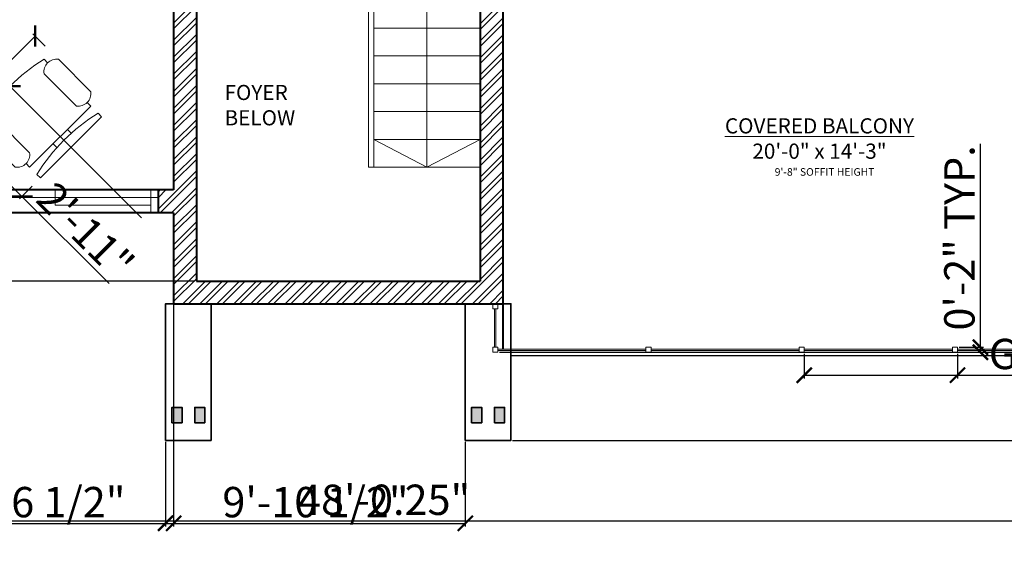
# Model space of a CAD drawing. Units: inches. Extents: x 982 to 1904, y 735 to 1463.
# Tile 2 of 7: x 1301 to 1689, y 735 to 945. Entities that reach past the tile are written whole.
import ezdxf

# ---------------------------------------------------------------- set-up
doc = ezdxf.new("R2010")
doc.units = ezdxf.units.IN
for name, color, linetype, lineweight in [('A-ANNO-TEXT', 7, 'Continuous', 18), ('A-AREA-IDEN', 7, 'Continuous', 18), ('A-COLS', 7, 'Continuous', 35), ('A-FLOR', 7, 'Continuous', 25), ('A-FLOR-RAIL', 7, 'Continuous', 18), ('Dimensions', 9, 'Continuous', 18), ('Furniture', 31, 'Continuous', 18), ('Stairs', 50, 'Continuous', 20), ('Wall Hatch', 23, 'Continuous', 13), ('Walls', 151, 'Continuous', 40), ('Windows', 111, 'Continuous', 18)]:
    doc.layers.add(name, color=color, linetype=linetype, lineweight=lineweight)
doc.layers.add('A-COLS-PATT', color=251, linetype='Continuous', lineweight=13, true_color=0x636466)
doc.styles.get("Standard").update_dxf_attribs({"font": 'arial.ttf'})
doc.dimstyles.new('ISO-25', dxfattribs={"dimtxt": 12, "dimasz": 6, "dimexe": 1.25, "dimexo": 0.625, "dimtad": 1, "dimlunit": 3, "dimtxsty": 'Standard', "dimblk": 'ARCHTICK', "dimcen": 2.5, "dimadec": 0, "dimazin": 0, "dimtfac": 1, "dimtmove": 0, "dimatfit": 3, "dimfxl": 1, "dimarcsym": 0})

# ---------------------------------------------------------------- blocks, each defined once
blk = doc.blocks.new('Chair - Desk')
for p, q in [((-8.5, 0), (-8.5, -1)), ((-8.5, 0), (8.5, 0)), ((8.5, 0), (8.5, -1)), ((-8.5, -3), (-8.5, -4)), ((-8.5, -3), (8.5, -3)), ((-2, -3), (-2, -1.9355)), ((2, -1.9576), (2, -3)), ((8.5, -3), (8.5, -4)), ((-10.5, -5), (-10.5, -14)), ((-6.5, -14), (-6.5, -5)), ((6.5, -5), (6.5, -14)), ((10.5, -14), (10.5, -5)), ((-8.5, -15), (-8.5, -16)), ((8.5, -15), (8.5, -16))]:
    blk.add_line(p, q)
for centre, radius, start, end in [((0, 34.625), 36.625, 256.5803, 283.4197), ((-8.5, -6.5), 2.5, 36.8699, 143.1301), ((8.5, -6.5), 2.5, 36.8699, 143.1301), ((-8.5, -12.5), 2.5, 216.8699, 323.1301), ((8.5, -12.5), 2.5, 216.8699, 323.1301), ((0, 19.625), 36.625, 256.5803, 283.4197)]:
    blk.add_arc(centre, radius, start, end)
blk = doc.blocks.new('_ArchTick')
at = {"color": 0, "linetype": 'ByBlock', "const_width": 0.15}
blk.add_lwpolyline([(-0.5, -0.5), (0.5, 0.5)], dxfattribs=at)
blk = doc.blocks.new('*D22')
at = {"layer": 'Defpoints', "color": 0, "transparency": 16777216}
for p in [(1156.5, 893.99), (1732.75, 812.49), (1732.75, 747.2)]:
    blk.add_point(p, dxfattribs=at)
at = {"layer": 'Dimensions', "color": 0, "lineweight": -2, "transparency": 16777216}
for p, q in [((1156.5, 893.37), (1156.5, 745.95)), ((1732.75, 811.87), (1732.75, 745.95)), ((1156.5, 747.2), (1732.75, 747.2))]:
    blk.add_line(p, q, dxfattribs=at)
at = {"layer": 'Dimensions', "color": 0, "lineweight": -2, "transparency": 16777216, "xscale": 6, "yscale": 6, "zscale": 6, "rotation": 180}
blk.add_blockref('_ArchTick', (1156.5, 747.2), dxfattribs=at)
at = {"layer": 'Dimensions', "color": 0, "lineweight": -2, "transparency": 16777216, "xscale": 6, "yscale": 6, "zscale": 6}
blk.add_blockref('_ArchTick', (1732.75, 747.2), dxfattribs=at)
at = {"layer": 'Dimensions', "color": 0, "transparency": 16777216, "insert": (1444.62, 753.95), "char_height": 12, "attachment_point": 5}
blk.add_mtext('48\'-0.25"', dxfattribs=at)
blk = doc.blocks.new('POST-BASE-18x54')
for points in [[(0, 0), (18, 0), (18, 54), (0, 54)], [(2.5, 7), (6.5, 7), (6.5, 13), (2.5, 13)], [(11.5, 7), (15.5, 7), (15.5, 13), (11.5, 13)]]:
    blk.add_lwpolyline(points, close=True)
blk = doc.blocks.new('GUARD-PANEL-60_5')
for p, q in [((0, 1.16), (58.5, 1.16)), ((0, 0.66), (58.5, 0.66))]:
    blk.add_line(p, q)
blk.add_lwpolyline([(58.5, 2), (60.5, 2), (60.5, 0), (58.5, 0)], close=True)
blk = doc.blocks.new('*D28')
at = {"layer": 'Defpoints', "color": 0, "transparency": 16777216}
for p in [(1610.5, 813.83), (1671, 813.83), (1671, 804.76)]:
    blk.add_point(p, dxfattribs=at)
at = {"layer": 'Dimensions', "color": 0, "lineweight": -2, "transparency": 16777216}
for p, q in [((1610.5, 813.21), (1610.5, 803.51)), ((1671, 813.21), (1671, 803.51)), ((1610.5, 804.76), (1671, 804.76)), ((1671, 804.76), (1903.99, 804.76))]:
    blk.add_line(p, q, dxfattribs=at)
at = {"layer": 'Dimensions', "color": 0, "lineweight": -2, "transparency": 16777216, "xscale": 6, "yscale": 6, "zscale": 6, "rotation": 180}
blk.add_blockref('_ArchTick', (1610.5, 804.76), dxfattribs=at)
at = {"layer": 'Dimensions', "color": 0, "lineweight": -2, "transparency": 16777216, "xscale": 6, "yscale": 6, "zscale": 6}
blk.add_blockref('_ArchTick', (1671, 804.76), dxfattribs=at)
at = {"layer": 'Dimensions', "color": 0, "transparency": 16777216, "insert": (1790.49, 811.59), "char_height": 12, "attachment_point": 5}
blk.add_mtext('GUARD PANEL 5\'-0 1/2" TYP.', dxfattribs=at)
blk = doc.blocks.new('*D29')
at = {"layer": 'Defpoints', "color": 0, "transparency": 16777216}
for p in [(1671, 815.83), (1671, 813.83), (1680.07, 815.83)]:
    blk.add_point(p, dxfattribs=at)
at = {"layer": 'Dimensions', "color": 0, "lineweight": -2, "transparency": 16777216}
for p, q in [((1680.07, 815.83), (1680.07, 896.23)), ((1671.62, 815.83), (1681.32, 815.83)), ((1671.62, 813.83), (1681.32, 813.83)), ((1680.07, 813.83), (1680.07, 815.83))]:
    blk.add_line(p, q, dxfattribs=at)
at = {"layer": 'Dimensions', "color": 0, "lineweight": -2, "transparency": 16777216, "xscale": 6, "yscale": 6, "zscale": 6}
for p, rotation in [((1680.07, 815.83), 90), ((1680.07, 813.83), 270)]:
    blk.add_blockref('_ArchTick', p, dxfattribs=dict(at, rotation=rotation))
at = {"layer": 'Dimensions', "color": 0, "transparency": 16777216, "insert": (1673.32, 859.03), "char_height": 12, "attachment_point": 5, "rotation": 90}
blk.add_mtext('0\'-2" TYP.', dxfattribs=at)
blk = doc.blocks.new('*D50')
at = {"layer": 'Defpoints', "color": 0, "transparency": 16777216}
for p in [(1311.27, 934.37), (1276.96, 909.01), (1281.43, 904.53)]:
    blk.add_point(p, dxfattribs=at)
at = {"layer": 'Dimensions', "color": 0, "lineweight": -2, "transparency": 16777216}
for p, q in [((1306.8, 938.85), (1276.96, 909.01)), ((1310.83, 934.81), (1305.91, 939.73)), ((1280.99, 904.97), (1276.07, 909.89)), ((1276.96, 909.01), (1173.95, 806))]:
    blk.add_line(p, q, dxfattribs=at)
at = {"layer": 'Dimensions', "color": 0, "lineweight": -2, "transparency": 16777216, "xscale": 6, "yscale": 6, "zscale": 6}
for p, rotation in [((1306.8, 938.85), 44.99970894708495), ((1276.96, 909.01), 224.9997089470849)]:
    blk.add_blockref('_ArchTick', p, dxfattribs=dict(at, rotation=rotation))
at = {"layer": 'Dimensions', "color": 0, "transparency": 16777216, "insert": (1218.5, 860.22), "char_height": 12, "attachment_point": 5, "rotation": 44.9997}
blk.add_mtext('DESK CHAIR 3\'-6"', dxfattribs=at)
blk = doc.blocks.new('*D51')
at = {"layer": 'Defpoints', "color": 0, "transparency": 16777216}
for p in [(1281.43, 904.53), (1306.06, 879.9), (1301.59, 875.42)]:
    blk.add_point(p, dxfattribs=at)
at = {"layer": 'Dimensions', "color": 0, "lineweight": -2, "transparency": 16777216}
for p, q in [((1280.99, 904.09), (1276.07, 899.17)), ((1276.96, 900.06), (1301.59, 875.42)), ((1305.62, 879.46), (1300.7, 874.54)), ((1301.59, 875.42), (1336.01, 841))]:
    blk.add_line(p, q, dxfattribs=at)
at = {"layer": 'Dimensions', "color": 0, "lineweight": -2, "transparency": 16777216, "xscale": 6, "yscale": 6, "zscale": 6}
for p, rotation in [((1276.96, 900.06), 134.9997089470847), ((1301.59, 875.42), 314.9997089470847)]:
    blk.add_blockref('_ArchTick', p, dxfattribs=dict(at, rotation=rotation))
at = {"layer": 'Dimensions', "color": 0, "transparency": 16777216, "insert": (1325.62, 860.8), "char_height": 12, "attachment_point": 5, "rotation": 314.9997}
blk.add_mtext('2\'-11"', dxfattribs=at)
blk = doc.blocks.new('*D54')
at = {"layer": 'Defpoints', "color": 0, "transparency": 16777216}
for p in [(1489.5, 813.83), (1769.32, 813.83), (1494.68, 778.99)]:
    blk.add_point(p, dxfattribs=at)
at = {"layer": 'Dimensions', "color": 0, "lineweight": -2, "transparency": 16777216}
for p, q in [((1769.32, 813.83), (1769.32, 862.51)), ((1490.12, 813.83), (1770.57, 813.83)), ((1769.32, 778.99), (1769.32, 813.83)), ((1495.3, 778.99), (1770.57, 778.99))]:
    blk.add_line(p, q, dxfattribs=at)
at = {"layer": 'Dimensions', "color": 0, "lineweight": -2, "transparency": 16777216, "xscale": 6, "yscale": 6, "zscale": 6}
for p, rotation in [((1769.32, 813.83), 90), ((1769.32, 778.99), 270)]:
    blk.add_blockref('_ArchTick', p, dxfattribs=dict(at, rotation=rotation))
at = {"layer": 'Dimensions', "color": 0, "transparency": 16777216, "insert": (1762.67, 841.17), "char_height": 12, "attachment_point": 5, "rotation": 90}
blk.add_mtext('2\'-11"', dxfattribs=at)
blk = doc.blocks.new('*D62')
at = {"layer": 'Defpoints', "color": 0, "transparency": 16777216}
for p in [(1259, 868.99), (1361.5, 868.99), (1361.5, 746.19)]:
    blk.add_point(p, dxfattribs=at)
at = {"layer": 'Dimensions', "color": 0, "lineweight": -2, "transparency": 16777216}
for p, q in [((1259, 868.37), (1259, 744.94)), ((1361.5, 868.37), (1361.5, 744.94)), ((1259, 746.19), (1361.5, 746.19))]:
    blk.add_line(p, q, dxfattribs=at)
at = {"layer": 'Dimensions', "color": 0, "lineweight": -2, "transparency": 16777216, "xscale": 6, "yscale": 6, "zscale": 6, "rotation": 180}
blk.add_blockref('_ArchTick', (1259, 746.19), dxfattribs=at)
at = {"layer": 'Dimensions', "color": 0, "lineweight": -2, "transparency": 16777216, "xscale": 6, "yscale": 6, "zscale": 6}
blk.add_blockref('_ArchTick', (1361.5, 746.19), dxfattribs=at)
at = {"layer": 'Dimensions', "color": 0, "transparency": 16777216, "insert": (1310.25, 753.02), "char_height": 12, "attachment_point": 5}
blk.add_mtext('8\'-6 1/2"', dxfattribs=at)
blk = doc.blocks.new('*D64')
at = {"layer": 'Defpoints', "color": 0, "transparency": 16777216}
for p in [(1482.5, 1427.79), (1370.5, 841.99), (1482.5, 841.99)]:
    blk.add_point(p, dxfattribs=at)
at = {"layer": 'Dimensions', "color": 0, "lineweight": -2, "transparency": 16777216}
for p, q in [((1370.5, 842.62), (1370.5, 1429.04)), ((1370.5, 1427.79), (1482.5, 1427.79)), ((1482.5, 842.62), (1482.5, 1429.04))]:
    blk.add_line(p, q, dxfattribs=at)
at = {"layer": 'Dimensions', "color": 0, "lineweight": -2, "transparency": 16777216, "xscale": 6, "yscale": 6, "zscale": 6, "rotation": 180}
blk.add_blockref('_ArchTick', (1370.5, 1427.79), dxfattribs=at)
at = {"layer": 'Dimensions', "color": 0, "lineweight": -2, "transparency": 16777216, "xscale": 6, "yscale": 6, "zscale": 6}
blk.add_blockref('_ArchTick', (1482.5, 1427.79), dxfattribs=at)
at = {"layer": 'Dimensions', "color": 0, "transparency": 16777216, "insert": (1426.5, 1434.54), "char_height": 12, "attachment_point": 5}
blk.add_mtext('9\'-4"', dxfattribs=at)
blk = doc.blocks.new('*D65')
at = {"layer": 'Defpoints', "color": 0, "transparency": 16777216}
for p in [(1123.7, 1042.99), (1370.5, 1042.99), (1370.5, 841.99)]:
    blk.add_point(p, dxfattribs=at)
at = {"layer": 'Dimensions', "color": 0, "lineweight": -2, "transparency": 16777216}
for p, q in [((1369.87, 1042.99), (1122.45, 1042.99)), ((1123.7, 841.99), (1123.7, 1042.99)), ((1369.87, 841.99), (1122.45, 841.99))]:
    blk.add_line(p, q, dxfattribs=at)
at = {"layer": 'Dimensions', "color": 0, "lineweight": -2, "transparency": 16777216, "xscale": 6, "yscale": 6, "zscale": 6}
for p, rotation in [((1123.7, 1042.99), 90), ((1123.7, 841.99), 270)]:
    blk.add_blockref('_ArchTick', p, dxfattribs=dict(at, rotation=rotation))
at = {"layer": 'Dimensions', "color": 0, "transparency": 16777216, "insert": (1116.94, 942.49), "char_height": 12, "attachment_point": 5, "rotation": 90}
blk.add_mtext('16\'-9"', dxfattribs=at)
blk = doc.blocks.new('*D71')
at = {"layer": 'Defpoints', "color": 0, "transparency": 16777216}
for p in [(1358.31, 778.99), (1476.68, 778.99), (1476.68, 746.19)]:
    blk.add_point(p, dxfattribs=at)
at = {"layer": 'Dimensions', "color": 0, "lineweight": -2, "transparency": 16777216}
for p, q in [((1358.31, 778.37), (1358.31, 744.94)), ((1476.68, 778.37), (1476.68, 744.94)), ((1358.31, 746.19), (1476.68, 746.19))]:
    blk.add_line(p, q, dxfattribs=at)
at = {"layer": 'Dimensions', "color": 0, "lineweight": -2, "transparency": 16777216, "xscale": 6, "yscale": 6, "zscale": 6, "rotation": 180}
blk.add_blockref('_ArchTick', (1358.31, 746.19), dxfattribs=at)
at = {"layer": 'Dimensions', "color": 0, "lineweight": -2, "transparency": 16777216, "xscale": 6, "yscale": 6, "zscale": 6}
blk.add_blockref('_ArchTick', (1476.68, 746.19), dxfattribs=at)
at = {"layer": 'Dimensions', "color": 0, "transparency": 16777216, "insert": (1417.5, 753.02), "char_height": 12, "attachment_point": 5}
blk.add_mtext('9\'-10 1/2"', dxfattribs=at)
blk = doc.blocks.new('*D75')
at = {"layer": 'Defpoints', "color": 0, "transparency": 16777216}
for p in [(1296.83, 918.98), (1348.87, 866.93)]:
    blk.add_point(p, dxfattribs=at)
at = {"layer": 'Dimensions', "color": 0, "lineweight": -2, "transparency": 16777216}
for p in [(1218.63, 997.17), (1348.87, 866.93)]:
    blk.add_line(p, (1296.83, 918.98), dxfattribs=at)
at = {"layer": 'Dimensions', "color": 0, "lineweight": -2, "transparency": 16777216, "xscale": 6, "yscale": 6, "zscale": 6, "rotation": 314.9994011111431}
blk.add_blockref('_ArchTick', (1296.83, 918.98), dxfattribs=at)
at = {"layer": 'Dimensions', "color": 0, "transparency": 16777216, "insert": (1258.32, 967.15), "char_height": 12, "attachment_point": 5, "rotation": 314.9994}
blk.add_mtext('2X R6\'-1 1/2"', dxfattribs=at)

msp = doc.modelspace()

# ---------------------------------------------------------------- hatches: boundary and pattern name
at = {"layer": 'A-COLS-PATT'}
h = msp.add_hatch(color=256, dxfattribs=at)
h.dxf.hatch_style = 1
h.paths.add_polyline_path([(1731.496, 1394.991), (1722.496, 1394.991), (1722.496, 1385.991), (1731.496, 1385.991)])
h.paths.add_polyline_path([(1725.019, 843.656), (1721.019, 843.656), (1721.019, 837.656), (1725.019, 837.656)])
h.paths.add_polyline_path([(1734.019, 843.656), (1730.019, 843.656), (1730.019, 837.656), (1734.019, 837.656)])
h.paths.add_polyline_path([(1483.18, 791.991), (1479.18, 791.991), (1479.18, 785.991), (1483.18, 785.991)])
h.paths.add_polyline_path([(1492.18, 791.991), (1488.18, 791.991), (1488.18, 785.991), (1492.18, 785.991)])
h.paths.add_polyline_path([(1364.813, 791.991), (1360.813, 791.991), (1360.813, 785.991), (1364.813, 785.991)])
h.paths.add_polyline_path([(1373.813, 791.991), (1369.813, 791.991), (1369.813, 785.991), (1373.813, 785.991)])
at = {"layer": 'Wall Hatch'}
h = msp.add_hatch(dxfattribs=at)
h.set_pattern_fill('ANSI32', color=256, scale=0.5)
h.paths.add_polyline_path([(1165.496, 1065.991), (1271.496, 1065.991), (1271.496, 1071.991), (1218.496, 1071.991), (1218.496, 1238.491), (1262.496, 1238.491), (1262.496, 1244.491), (1218.496, 1244.491), (1218.496, 1330.491), (1298.496, 1330.491), (1298.496, 1244.491), (1292.496, 1244.491), (1292.496, 1238.491), (1298.496, 1238.491), (1298.496, 1221.991), (1304.496, 1221.991), (1304.496, 1224.991), (1374.496, 1224.991), (1374.496, 1230.991), (1304.496, 1230.991), (1304.496, 1251.991), (1310.496, 1251.991), (1310.496, 1257.991), (1304.496, 1257.991), (1304.496, 1385.991), (1328.496, 1385.991), (1328.496, 1394.991), (1295.496, 1394.991), (1295.496, 1339.491), (1209.496, 1339.491), (1209.496, 1071.991), (1156.496, 1071.991), (1156.496, 893.991), (1171.496, 893.991), (1171.496, 902.991), (1165.496, 902.991)])
h.paths.add_polyline_path([(1273.996, 877.991), (1267.996, 877.991), (1267.996, 902.991), (1252.996, 902.991), (1252.996, 893.991), (1258.996, 893.991), (1258.996, 868.991), (1273.996, 868.991)])
h.paths.add_polyline_path([(1370.496, 1052.991), (1361.496, 1052.991), (1361.496, 1046.991), (1355.496, 1046.991), (1355.496, 1040.991), (1361.496, 1040.991), (1361.496, 877.991), (1355.496, 877.991), (1355.496, 868.991), (1361.496, 868.991), (1361.496, 832.991), (1376.313, 832.991), (1491.496, 832.991), (1491.496, 985.991), (1515.496, 985.991), (1515.496, 994.991), (1482.496, 994.991), (1482.496, 841.991), (1370.496, 841.991)])
h.paths.add_polyline_path([(1319.496, 1088.991), (1325.496, 1088.991), (1325.496, 1094.991), (1319.496, 1094.991), (1319.496, 1112.491), (1361.496, 1112.491), (1361.496, 1094.991), (1355.496, 1094.991), (1355.496, 1088.991), (1361.496, 1088.991), (1361.496, 1082.991), (1370.496, 1082.991), (1370.496, 1180.991), (1503.496, 1180.991), (1503.496, 1231.991), (1497.496, 1231.991), (1497.496, 1215.991), (1491.496, 1215.991), (1491.496, 1209.991), (1497.496, 1209.991), (1497.496, 1189.991), (1448.496, 1189.991), (1448.496, 1209.991), (1454.496, 1209.991), (1454.496, 1215.991), (1448.496, 1215.991), (1448.496, 1221.991), (1442.496, 1221.991), (1442.496, 1189.991), (1380.496, 1189.991), (1380.496, 1251.991), (1442.496, 1251.991), (1442.496, 1245.991), (1448.496, 1245.991), (1448.496, 1263.991), (1442.496, 1263.991), (1442.496, 1257.991), (1368.496, 1257.991), (1368.496, 1251.991), (1374.496, 1251.991), (1374.496, 1189.991), (1304.496, 1189.991), (1304.496, 1192.991), (1295.496, 1192.991), (1295.496, 1183.991), (1361.496, 1183.991), (1361.496, 1118.491), (1313.496, 1118.491), (1313.496, 1071.991), (1301.496, 1071.991), (1301.496, 1065.991), (1313.496, 1065.991), (1313.496, 1040.991), (1325.496, 1040.991), (1325.496, 1046.991), (1319.496, 1046.991)])
h.paths.add_polyline_path([(1565.496, 1394.991), (1418.496, 1394.991), (1418.496, 1385.991), (1442.496, 1385.991), (1442.496, 1293.991), (1448.496, 1293.991), (1448.496, 1299.991), (1454.496, 1299.991), (1454.496, 1305.991), (1448.496, 1305.991), (1448.496, 1385.991), (1556.496, 1385.991), (1556.496, 1307.991), (1497.496, 1307.991), (1497.496, 1305.991), (1491.496, 1305.991), (1491.496, 1299.991), (1497.496, 1299.991), (1497.496, 1268.991), (1503.496, 1268.991), (1503.496, 1298.991), (1656.496, 1298.991), (1656.496, 1307.991), (1565.496, 1307.991)])
h.paths.add_polyline_path([(1731.496, 1307.991), (1698.496, 1307.991), (1698.496, 1298.991), (1722.496, 1298.991), (1722.496, 1033.991), (1731.496, 1033.991)])
h.paths.add_polyline_path([(1731.496, 997.991), (1722.496, 997.991), (1722.496, 994.991), (1689.496, 994.991), (1689.496, 985.991), (1731.496, 985.991)])

# ---------------------------------------------------------------- linework, layer by layer
at = {"layer": 'A-FLOR'}
msp.add_line((1494.68, 812.491), (1732.746, 812.491), dxfattribs=at)
at = {"layer": 'A-FLOR-RAIL'}
for p, q in [((1488.246, 830.991), (1488.246, 815.833)), ((1488.746, 830.991), (1488.746, 815.833))]:
    msp.add_line(p, q, dxfattribs=at)
for points in [[(1487.496, 830.991), (1489.496, 830.991), (1489.496, 832.991), (1487.496, 832.991)], [(1487.496, 815.833), (1489.496, 815.833), (1489.496, 813.833), (1487.496, 813.833)]]:
    msp.add_lwpolyline(points, close=True, dxfattribs=at)
at = {"layer": 'Stairs'}
for p, q in [((1438.496, 1043.012), (1438.496, 886.991)), ((1440.496, 1043.012), (1440.496, 886.991)), ((1461.496, 886.991), (1461.496, 1043.019)), ((1440.496, 941.991), (1482.496, 941.991)), ((1440.496, 930.991), (1482.496, 930.991)), ((1440.496, 919.991), (1482.496, 919.991)), ((1440.496, 908.991), (1482.496, 908.991)), ((1440.496, 897.991), (1482.496, 897.991)), ((1440.496, 897.991), (1461.496, 886.991)), ((1461.496, 886.991), (1482.496, 897.991)), ((1438.496, 886.991), (1482.496, 886.991))]:
    msp.add_line(p, q, dxfattribs=at)
at = {"layer": 'Walls'}
for p, q in [((1370.496, 1052.991), (1370.496, 841.991)), ((1482.496, 1043.025), (1482.496, 841.991)), ((1361.496, 1040.991), (1361.496, 877.991)), ((1491.496, 985.991), (1491.496, 814.991)), ((1361.496, 877.991), (1267.996, 877.991)), ((1355.496, 868.991), (1355.496, 877.991)), ((1361.496, 868.991), (1258.996, 868.991)), ((1361.496, 868.991), (1361.496, 832.991)), ((1370.496, 841.991), (1482.496, 841.991)), ((1361.496, 832.991), (1491.496, 832.991))]:
    msp.add_line(p, q, dxfattribs=at)
at = {"layer": 'Windows'}
for p, q in [((1355.496, 874.991), (1273.996, 874.991)), ((1314.746, 877.991), (1314.746, 871.991)), ((1352.496, 868.991), (1352.496, 877.991)), ((1352.496, 871.991), (1314.746, 871.991))]:
    msp.add_line(p, q, dxfattribs=at)

# ---------------------------------------------------------------- block references
at = {"layer": 'A-COLS', "extrusion": (0, 0, -1), "zscale": -1}
msp.add_blockref('POST-BASE-18x54', (-1376.313, 778.991), dxfattribs=at)
at = {"layer": 'A-COLS'}
msp.add_blockref('POST-BASE-18x54', (1476.68, 778.991), dxfattribs=at)
at = {"layer": 'A-FLOR-RAIL'}
for p in [(1489.496, 813.833), (1549.996, 813.833), (1610.496, 813.833), (1670.996, 813.833)]:
    msp.add_blockref('GUARD-PANEL-60_5', p, dxfattribs=at)
at = {"layer": 'Furniture', "xscale": 2.009614080572303, "yscale": 2.009614080572303, "zscale": 2.009614080572303, "rotation": 224.9997089470848}
msp.add_blockref('Chair - Desk', (1320.983, 894.821), dxfattribs=at)

# ---------------------------------------------------------------- texts
at = {"layer": 'A-ANNO-TEXT', "insert": (1575.903, 886.614), "char_height": 3, "attachment_point": 1}
msp.add_mtext_dynamic_manual_height_columns('\\pxqc;{\\fTimes New Roman|b0|i0|c0|p18;\\T1.25;9\'-8" SOFFIT HEIGHT}', width=85.22884, gutter_width=12.5, heights=[0], dxfattribs=at)
at = {"layer": 'A-AREA-IDEN', "char_height": 6, "attachment_point": 1}
for s, width, insert in [('{\\fTimes New Roman|b0|i0|c0|p18;FOYER BELOW}', 41.80763, (1381.603, 919.526)), ('\\pxqc;{\\fTimes New Roman|b0|i0|c0|p18;\\LCOVERED BALCONY\\P\\l20\'-0" x 14\'-3"}', 97.93162, (1567.548, 906.326))]:
    msp.add_mtext_dynamic_manual_height_columns(s, width=width, gutter_width=12.5, heights=[0], dxfattribs=dict(at, insert=insert))

# ---------------------------------------------------------------- dimensions: what is measured, and where the dimension line sits
at = {"layer": 'Dimensions'}
for base, p1, p2, override, picture, middle in [((1482.496, 1427.791), (1370.496, 841.991), (1482.496, 841.991), {"dimdec": 1, "dimlfac": 1, "dimrnd": 0, "dimzin": 1, "dimdsep": 46, "dimlunit": 4, "dimfrac": 2}, '*D64', (1426.496, 1434.543)), ((1732.746, 747.196), (1156.496, 893.991), (1732.746, 812.491), {"dimclrd": 0, "dimclre": 0, "dimclrt": 0}, '*D22', (1444.621, 753.948)), ((1361.496, 746.191), (1258.996, 868.991), (1361.496, 868.991), {"dimdec": 1, "dimlfac": 1, "dimrnd": 0, "dimzin": 1, "dimdsep": 46, "dimlunit": 4, "dimfrac": 2}, '*D62', (1310.246, 753.021)), ((1476.68, 746.191), (1358.313, 778.991), (1476.68, 778.991), {"dimdec": 1, "dimlfac": 1, "dimrnd": 0, "dimzin": 1, "dimdsep": 46, "dimlunit": 4, "dimfrac": 2}, '*D71', (1417.496, 753.021))]:
    dim = msp.add_linear_dim(base=base, p1=p1, p2=p2, dimstyle='ISO-25', override=override, dxfattribs=at)
    dim.commit()
    dim.dimension.update_dxf_attribs({"geometry": picture, "text_midpoint": middle})
for base, p1, p2, angle, picture, middle in [((1123.696, 1042.991), (1370.496, 841.991), (1370.496, 1042.991), 90, '*D65', (1116.945, 942.491)), ((1301.586, 875.425), (1281.431, 904.532), (1306.062, 879.901), 314.99971, '*D51', (1325.619, 860.795)), ((1769.319, 813.833), (1494.68, 778.991), (1489.496, 813.833), 90, '*D54', (1762.669, 841.172))]:
    dim = msp.add_linear_dim(base=base, p1=p1, p2=p2, angle=angle, dimstyle='ISO-25', override={"dimdec": 1, "dimlfac": 1, "dimrnd": 0, "dimzin": 1, "dimdsep": 46, "dimlunit": 4, "dimfrac": 2}, dxfattribs=at)
    dim.commit()
    dim.dimension.update_dxf_attribs({"geometry": picture, "text_midpoint": middle})
dim = msp.add_radius_dim(center=(1348.87, 866.934), mpoint=(1296.826, 918.979), text='2X <>', dimstyle='ISO-25', override={"dimdec": 1, "dimlfac": 1, "dimrnd": 0, "dimzin": 1, "dimdsep": 46, "dimlunit": 4, "dimfrac": 2}, dxfattribs=at)
dim.commit()
dim.dimension.update_dxf_attribs({"geometry": '*D75', "text_midpoint": (1258.316, 967.149)})
for base, p1, p2, angle, text, picture, middle in [((1276.955, 909.008), (1311.273, 934.373), (1281.431, 904.532), 224.99971, 'DESK CHAIR <>', '*D50', (1218.497, 860.215)), ((1680.071, 815.833), (1670.996, 813.833), (1670.996, 815.833), 90, '<> TYP.', '*D29', (1673.32, 859.031))]:
    dim = msp.add_linear_dim(base=base, p1=p1, p2=p2, angle=angle, text=text, dimstyle='ISO-25', override={"dimdec": 1, "dimlfac": 1, "dimrnd": 0, "dimzin": 1, "dimdsep": 46, "dimlunit": 4, "dimfrac": 2}, dxfattribs=at)
    dim.commit()
    dim.dimension.update_dxf_attribs({"geometry": picture, "text_midpoint": middle})
dim = msp.add_linear_dim(base=(1670.996, 804.758), p1=(1610.496, 813.833), p2=(1670.996, 813.833), text='GUARD PANEL <> TYP.', dimstyle='ISO-25', override={"dimdec": 1, "dimlfac": 1, "dimrnd": 0, "dimzin": 1, "dimdsep": 46, "dimlunit": 4, "dimfrac": 2}, dxfattribs=at)
dim.commit()
dim.dimension.update_dxf_attribs({"geometry": '*D28', "text_midpoint": (1790.492, 811.588)})

doc.saveas('drawing.dxf')
